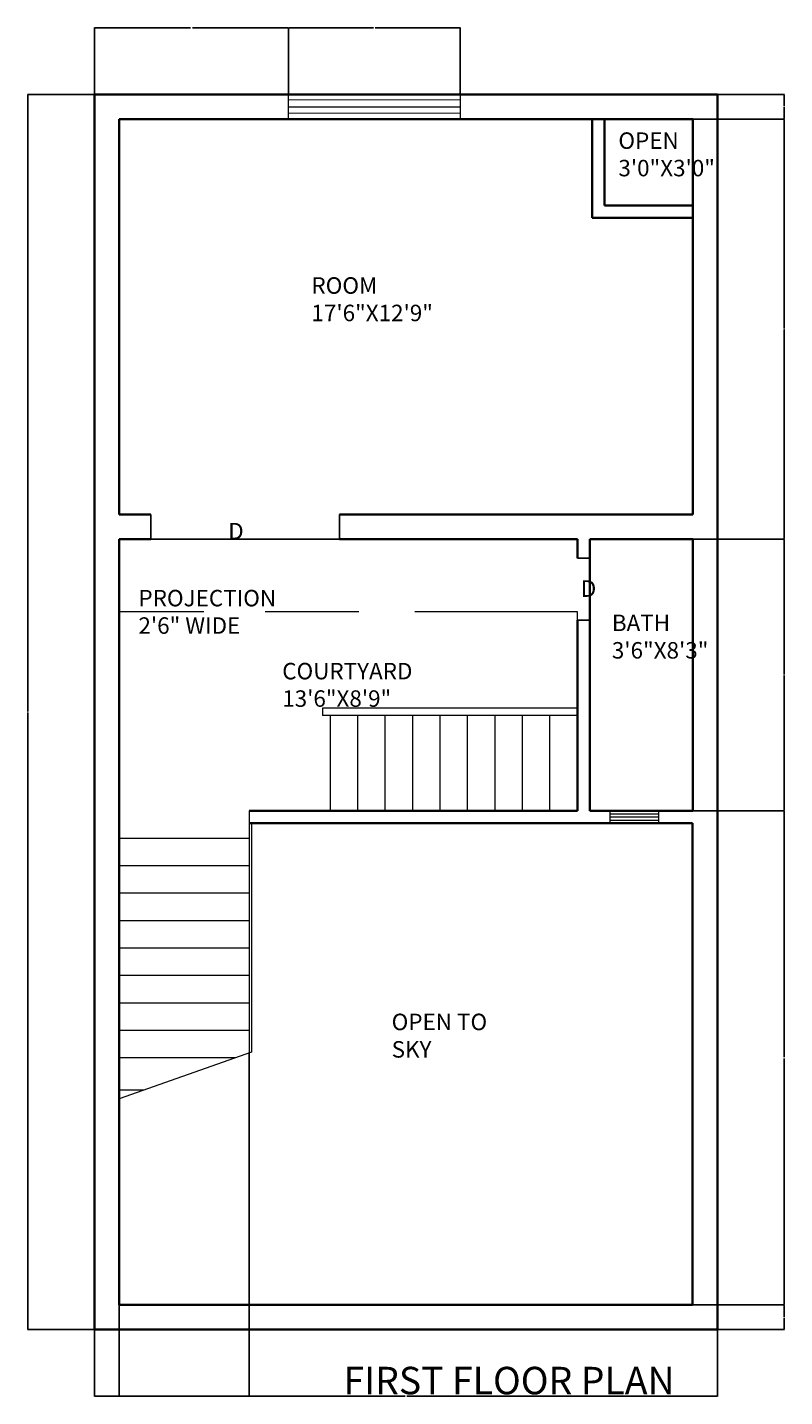
# Model space of a CAD drawing. Units: inches. Extents: x 2673 to 3344, y 1818 to 2362.
# Tile 2 of 2: x 3068 to 3344, y 1819 to 2318. Entities that reach past the tile are written whole.
import ezdxf

# ---------------------------------------------------------------- set-up
doc = ezdxf.new("R2010")
doc.units = ezdxf.units.IN
for name, color, linetype, lineweight in [('A-ANNO-DIMS', 2, 'Continuous', 18), ('A-ANNO-TEXT', 7, 'Continuous', 18), ('A-ANNO-TITL', 7, 'Continuous', 35), ('A-AREA-IDEN', 7, 'Continuous', 18), ('A-DOOR', 3, 'Continuous', 25), ('A-FLOR-PROJ', 8, 'Continuous', 13), ('A-FLOR-STRS', 8, 'Continuous', 18), ('A-GLAZ', 4, 'Continuous', 18), ('A-WALL', 7, 'Continuous', 35)]:
    doc.layers.add(name, color=color, linetype=linetype, lineweight=lineweight)
doc.styles.get("Standard").update_dxf_attribs({"font": 'arial.ttf'})
doc.dimstyles.get("Standard").update_dxf_attribs({"dimtxt": 0.18, "dimasz": 0.18, "dimexe": 0.18, "dimexo": 0.0625, "dimgap": 0.09, "dimtad": 0, "dimtih": 1, "dimtoh": 1, "dimdec": 4, "dimzin": 0, "dimdsep": 46, "dimtxsty": 'Standard', "dimcen": 0.09, "dimadec": 0, "dimazin": 0, "dimtfac": 1, "dimtdec": 4, "dimtofl": 0, "dimtmove": 0, "dimatfit": 3, "dimfxl": 1, "dimtolj": 1, "dimtzin": 0, "dimarcsym": 0})

# ---------------------------------------------------------------- blocks, each defined once
blk = doc.blocks.new('FLOOR-PERIMETER-227X450')
for p, q in [((0, 450), (227, 450)), ((0, 0), (0, 450)), ((227, 450), (227, 0)), ((227, 0), (0, 0))]:
    blk.add_line(p, q)
blk = doc.blocks.new('*D4')
at = {"layer": 'A-ANNO-DIMS', "color": 0, "lineweight": -2, "transparency": 16777216}
for p, q in [((3092.08, 1843.73), (3092.08, 1819.36)), ((3319.08, 1843.73), (3319.08, 1819.36)), ((3092.26, 1819.54), (3205.29, 1819.54)), ((3318.9, 1819.54), (3205.87, 1819.54))]:
    blk.add_line(p, q, dxfattribs=at)
at = {"layer": 'A-ANNO-DIMS', "color": 0, "transparency": 16777216}
for points in [[(3092.26, 1819.57), (3092.26, 1819.51), (3092.08, 1819.54)], [(3318.9, 1819.57), (3318.9, 1819.51), (3319.08, 1819.54)]]:
    blk.add_solid(points, dxfattribs=at)
at = {"layer": 'Defpoints', "color": 0, "transparency": 16777216}
for p in [(3092.08, 1843.79), (3319.08, 1843.79), (3319.08, 1819.54)]:
    blk.add_point(p, dxfattribs=at)
at = {"layer": 'A-ANNO-DIMS', "color": 0, "transparency": 16777216, "insert": (3205.58, 1819.54), "char_height": 0.18, "attachment_point": 5}
blk.add_mtext('\\A1;227', dxfattribs=at)
blk = doc.blocks.new('*D5')
at = {"layer": 'A-ANNO-DIMS', "color": 0, "lineweight": -2, "transparency": 16777216}
for p, q in [((3092.02, 2293.79), (3067.65, 2293.79)), ((3067.83, 2293.61), (3067.83, 2068.98)), ((3067.83, 1843.97), (3067.83, 2068.61)), ((3092.02, 1843.79), (3067.65, 1843.79))]:
    blk.add_line(p, q, dxfattribs=at)
at = {"layer": 'A-ANNO-DIMS', "color": 0, "transparency": 16777216}
for points in [[(3067.8, 2293.61), (3067.86, 2293.61), (3067.83, 2293.79)], [(3067.8, 1843.97), (3067.86, 1843.97), (3067.83, 1843.79)]]:
    blk.add_solid(points, dxfattribs=at)
at = {"layer": 'Defpoints', "color": 0, "transparency": 16777216}
for p in [(3067.83, 2293.79), (3092.08, 2293.79), (3092.08, 1843.79)]:
    blk.add_point(p, dxfattribs=at)
at = {"layer": 'A-ANNO-DIMS', "color": 0, "transparency": 16777216, "insert": (3067.83, 2068.79), "char_height": 0.18, "attachment_point": 5}
blk.add_mtext('\\A1;450', dxfattribs=at)
blk = doc.blocks.new('*D22')
at = {"layer": 'A-ANNO-DIMS', "color": 0, "lineweight": -2, "transparency": 16777216}
for p, q in [((3148.4, 1944.47), (3148.4, 1819.36)), ((3101.08, 1927.78), (3101.08, 1819.36)), ((3101.26, 1819.54), (3124.35, 1819.54)), ((3148.22, 1819.54), (3125.14, 1819.54))]:
    blk.add_line(p, q, dxfattribs=at)
at = {"layer": 'A-ANNO-DIMS', "color": 0, "transparency": 16777216}
for points in [[(3101.26, 1819.57), (3101.26, 1819.51), (3101.08, 1819.54)], [(3148.22, 1819.57), (3148.22, 1819.51), (3148.4, 1819.54)]]:
    blk.add_solid(points, dxfattribs=at)
at = {"layer": 'Defpoints', "color": 0, "transparency": 16777216}
for p in [(3148.4, 1944.54), (3101.08, 1927.84), (3148.4, 1819.54)]:
    blk.add_point(p, dxfattribs=at)
at = {"layer": 'A-ANNO-DIMS', "color": 0, "transparency": 16777216, "insert": (3124.74, 1819.54), "char_height": 0.18, "attachment_point": 5}
blk.add_mtext('\\A1;47.32', dxfattribs=at)
blk = doc.blocks.new('*D23')
at = {"layer": 'A-ANNO-DIMS', "color": 0, "lineweight": -2, "transparency": 16777216}
for p, q in [((3310.09, 1852.79), (3343.51, 1852.79)), ((3343.33, 1852.61), (3343.33, 1848.48)), ((3343.33, 1843.97), (3343.33, 1848.11)), ((3319.14, 1843.79), (3343.51, 1843.79))]:
    blk.add_line(p, q, dxfattribs=at)
at = {"layer": 'A-ANNO-DIMS', "color": 0, "transparency": 16777216}
for points in [[(3343.3, 1852.61), (3343.36, 1852.61), (3343.33, 1852.79)], [(3343.3, 1843.97), (3343.36, 1843.97), (3343.33, 1843.79)]]:
    blk.add_solid(points, dxfattribs=at)
at = {"layer": 'Defpoints', "color": 0, "transparency": 16777216}
for p in [(3310.03, 1852.79), (3343.33, 1852.79), (3319.08, 1843.79)]:
    blk.add_point(p, dxfattribs=at)
at = {"layer": 'A-ANNO-DIMS', "color": 0, "transparency": 16777216, "insert": (3343.33, 1848.29), "char_height": 0.18, "attachment_point": 5}
blk.add_mtext('\\A1;9', dxfattribs=at)
blk = doc.blocks.new('*D24')
at = {"layer": 'A-ANNO-DIMS', "color": 0, "lineweight": -2, "transparency": 16777216}
for p, q in [((3310.14, 2032.8), (3343.51, 2032.8)), ((3343.33, 2032.62), (3343.33, 1942.98)), ((3343.33, 1852.97), (3343.33, 1942.61)), ((3310.09, 1852.79), (3343.51, 1852.79))]:
    blk.add_line(p, q, dxfattribs=at)
at = {"layer": 'A-ANNO-DIMS', "color": 0, "transparency": 16777216}
for points in [[(3343.3, 2032.62), (3343.36, 2032.62), (3343.33, 2032.8)], [(3343.3, 1852.97), (3343.36, 1852.97), (3343.33, 1852.79)]]:
    blk.add_solid(points, dxfattribs=at)
at = {"layer": 'Defpoints', "color": 0, "transparency": 16777216}
for p in [(3310.08, 2032.8), (3343.33, 2032.8), (3310.03, 1852.79)]:
    blk.add_point(p, dxfattribs=at)
at = {"layer": 'A-ANNO-DIMS', "color": 0, "transparency": 16777216, "insert": (3343.33, 1942.8), "char_height": 0.18, "attachment_point": 5}
blk.add_mtext('\\A1;180', dxfattribs=at)
blk = doc.blocks.new('*D25')
at = {"layer": 'A-ANNO-DIMS', "color": 0, "lineweight": -2, "transparency": 16777216}
for p, q in [((3310.14, 2131.8), (3343.51, 2131.8)), ((3343.33, 2131.62), (3343.33, 2082.48)), ((3343.33, 2032.98), (3343.33, 2082.12)), ((3310.14, 2032.8), (3343.51, 2032.8))]:
    blk.add_line(p, q, dxfattribs=at)
at = {"layer": 'A-ANNO-DIMS', "color": 0, "transparency": 16777216}
for points in [[(3343.3, 2131.62), (3343.36, 2131.62), (3343.33, 2131.8)], [(3343.3, 2032.98), (3343.36, 2032.98), (3343.33, 2032.8)]]:
    blk.add_solid(points, dxfattribs=at)
at = {"layer": 'Defpoints', "color": 0, "transparency": 16777216}
for p in [(3310.08, 2131.8), (3343.33, 2131.8), (3310.08, 2032.8)]:
    blk.add_point(p, dxfattribs=at)
at = {"layer": 'A-ANNO-DIMS', "color": 0, "transparency": 16777216, "insert": (3343.33, 2082.3), "char_height": 0.18, "attachment_point": 5}
blk.add_mtext('\\A1;99', dxfattribs=at)
blk = doc.blocks.new('*D26')
at = {"layer": 'A-ANNO-DIMS', "color": 0, "lineweight": -2, "transparency": 16777216}
for p, q in [((3310.14, 2284.79), (3343.51, 2284.79)), ((3343.33, 2284.61), (3343.33, 2208.48)), ((3343.33, 2131.98), (3343.33, 2208.11)), ((3310.14, 2131.8), (3343.51, 2131.8))]:
    blk.add_line(p, q, dxfattribs=at)
at = {"layer": 'A-ANNO-DIMS', "color": 0, "transparency": 16777216}
for points in [[(3343.3, 2284.61), (3343.36, 2284.61), (3343.33, 2284.79)], [(3343.3, 2131.98), (3343.36, 2131.98), (3343.33, 2131.8)]]:
    blk.add_solid(points, dxfattribs=at)
at = {"layer": 'Defpoints', "color": 0, "transparency": 16777216}
for p in [(3310.08, 2284.79), (3343.33, 2284.79), (3310.08, 2131.8)]:
    blk.add_point(p, dxfattribs=at)
at = {"layer": 'A-ANNO-DIMS', "color": 0, "transparency": 16777216, "insert": (3343.33, 2208.3), "char_height": 0.18, "attachment_point": 5}
blk.add_mtext('\\A1;153', dxfattribs=at)
blk = doc.blocks.new('*D27')
at = {"layer": 'A-ANNO-DIMS', "color": 0, "lineweight": -2, "transparency": 16777216}
for p, q in [((3319.14, 2293.79), (3343.51, 2293.79)), ((3343.33, 2293.61), (3343.33, 2289.48)), ((3310.14, 2284.79), (3343.51, 2284.79)), ((3343.33, 2284.97), (3343.33, 2289.11))]:
    blk.add_line(p, q, dxfattribs=at)
at = {"layer": 'A-ANNO-DIMS', "color": 0, "transparency": 16777216}
for points in [[(3343.3, 2293.61), (3343.36, 2293.61), (3343.33, 2293.79)], [(3343.3, 2284.97), (3343.36, 2284.97), (3343.33, 2284.79)]]:
    blk.add_solid(points, dxfattribs=at)
at = {"layer": 'Defpoints', "color": 0, "transparency": 16777216}
for p in [(3319.08, 2293.79), (3343.33, 2293.79), (3310.08, 2284.79)]:
    blk.add_point(p, dxfattribs=at)
at = {"layer": 'A-ANNO-DIMS', "color": 0, "transparency": 16777216, "insert": (3343.33, 2289.29), "char_height": 0.18, "attachment_point": 5}
blk.add_mtext('\\A1;9', dxfattribs=at)
blk = doc.blocks.new('*D28')
at = {"layer": 'A-ANNO-DIMS', "color": 0, "lineweight": -2, "transparency": 16777216}
for p, q in [((3092.08, 2293.86), (3092.08, 2318.22)), ((3092.26, 2318.04), (3127.03, 2318.04)), ((3162.58, 2318.04), (3127.82, 2318.04)), ((3162.76, 2293.86), (3162.76, 2318.22))]:
    blk.add_line(p, q, dxfattribs=at)
at = {"layer": 'A-ANNO-DIMS', "color": 0, "transparency": 16777216}
for points in [[(3092.26, 2318.07), (3092.26, 2318.01), (3092.08, 2318.04)], [(3162.58, 2318.07), (3162.58, 2318.01), (3162.76, 2318.04)]]:
    blk.add_solid(points, dxfattribs=at)
at = {"layer": 'Defpoints', "color": 0, "transparency": 16777216}
for p in [(3162.76, 2318.04), (3092.08, 2293.79), (3162.76, 2293.79)]:
    blk.add_point(p, dxfattribs=at)
at = {"layer": 'A-ANNO-DIMS', "color": 0, "transparency": 16777216, "insert": (3127.42, 2318.04), "char_height": 0.18, "attachment_point": 5}
blk.add_mtext('\\A1;70.68', dxfattribs=at)
blk = doc.blocks.new('*D29')
at = {"layer": 'A-ANNO-DIMS', "color": 0, "lineweight": -2, "transparency": 16777216}
for p, q in [((3162.76, 2293.86), (3162.76, 2318.22)), ((3162.94, 2318.04), (3193.74, 2318.04)), ((3225.18, 2318.04), (3194.39, 2318.04)), ((3225.36, 2293.86), (3225.36, 2318.22))]:
    blk.add_line(p, q, dxfattribs=at)
at = {"layer": 'A-ANNO-DIMS', "color": 0, "transparency": 16777216}
for points in [[(3162.94, 2318.07), (3162.94, 2318.01), (3162.76, 2318.04)], [(3225.18, 2318.07), (3225.18, 2318.01), (3225.36, 2318.04)]]:
    blk.add_solid(points, dxfattribs=at)
at = {"layer": 'Defpoints', "color": 0, "transparency": 16777216}
for p in [(3225.36, 2318.04), (3162.76, 2293.79), (3225.36, 2293.79)]:
    blk.add_point(p, dxfattribs=at)
at = {"layer": 'A-ANNO-DIMS', "color": 0, "transparency": 16777216, "insert": (3194.06, 2318.04), "char_height": 0.18, "attachment_point": 5}
blk.add_mtext('\\A1;62.6', dxfattribs=at)

msp = doc.modelspace()

# ---------------------------------------------------------------- linework, layer by layer
at = {"layer": 'A-DOOR'}
for p, q in [((3112.6344, 2131.7995), (3112.6344, 2140.7995)), ((3181.3427, 2131.7995), (3181.3427, 2140.7995)), ((3112.6344, 2131.7995), (3181.3427, 2131.7995)), ((3268.0279, 2124.8843), (3272.5279, 2124.8843)), ((3268.0279, 2102.2017), (3272.5279, 2102.2017))]:
    msp.add_line(p, q, dxfattribs=at)
at = {"layer": 'A-FLOR-PROJ'}
for p, q in [((3131.8694, 2105.3455), (3101.0804, 2105.3455)), ((3188.3899, 2105.3455), (3154.3017, 2105.3455)), ((3237.0736, 2105.3455), (3208.8429, 2105.3455)), ((3268.0279, 2105.3455), (3237.0736, 2105.3455)), ((3268.0279, 2102.2017), (3268.0279, 2105.3455))]:
    msp.add_line(p, q, dxfattribs=at)
at = {"layer": 'A-FLOR-STRS'}
for p, q in [((3268.0279, 2070.1486), (3175.14, 2070.1486)), ((3175.14, 2070.1486), (3175.14, 2067.5006)), ((3268.0279, 2067.5006), (3175.14, 2067.5006)), ((3178.0279, 2032.7995), (3178.0279, 2067.5006)), ((3188.0279, 2032.7995), (3188.0279, 2067.5006)), ((3198.0279, 2032.7995), (3198.0279, 2067.5006)), ((3208.0279, 2032.7995), (3208.0279, 2067.5006)), ((3218.0279, 2032.7995), (3218.0279, 2067.5006)), ((3228.0279, 2032.7995), (3228.0279, 2067.5006)), ((3238.0279, 2032.7995), (3238.0279, 2067.5006)), ((3248.0279, 2032.7995), (3248.0279, 2067.5006)), ((3258.0279, 2032.7995), (3258.0279, 2067.5006)), ((3148.4041, 2032.7995), (3148.4041, 1944.5366)), ((3149.2926, 2028.2995), (3149.2926, 1944.85)), ((3148.4041, 2022.7553), (3101.0804, 2022.7553)), ((3148.4041, 2012.7553), (3101.0804, 2012.7553)), ((3148.4041, 2002.7553), (3101.0804, 2002.7553)), ((3148.4041, 1992.7553), (3101.0804, 1992.7553)), ((3148.4041, 1982.7553), (3101.0804, 1982.7553)), ((3148.4041, 1972.7553), (3101.0804, 1972.7553)), ((3148.4041, 1962.7553), (3101.0804, 1962.7553)), ((3148.4041, 1952.7553), (3101.0804, 1952.7553)), ((3149.2926, 1944.85), (3101.0804, 1927.8425)), ((3143.3545, 1942.7553), (3101.0804, 1942.7553)), ((3110.1895, 1931.0558), (3101.0804, 1931.0558))]:
    msp.add_line(p, q, dxfattribs=at)
at = {"layer": 'A-GLAZ'}
for p, q in [((3162.7644, 2291.8686), (3225.363, 2291.93)), ((3162.7644, 2289.2936), (3225.363, 2289.2936)), ((3162.7644, 2286.9977), (3225.363, 2287.0505)), ((3279.9327, 2031.7014), (3297.5645, 2031.7014)), ((3279.9327, 2030.5495), (3297.5645, 2030.5495)), ((3279.9327, 2029.387), (3297.5645, 2029.387))]:
    msp.add_line(p, q, dxfattribs=at)
for points in [[(3162.7644, 2293.7936), (3225.363, 2293.7936), (3225.363, 2284.7936), (3162.7644, 2284.7936)], [(3279.9327, 2032.7995), (3297.5645, 2032.7995), (3297.5645, 2028.2995), (3279.9327, 2028.2995)]]:
    msp.add_lwpolyline(points, close=True, dxfattribs=at)
at = {"layer": 'A-WALL'}
for p, q in [((3101.0804, 2284.7936), (3310.0804, 2284.7936)), ((3101.0804, 2140.7995), (3101.0804, 2284.7936)), ((3273.4559, 2248.799), (3273.4559, 2284.7936)), ((3277.9559, 2253.299), (3277.9559, 2284.7936)), ((3310.0804, 2284.7936), (3310.0804, 2140.7995)), ((3309.4559, 2253.299), (3277.9559, 2253.299)), ((3309.4559, 2253.299), (3310.0804, 2253.299)), ((3309.4559, 2248.799), (3273.4559, 2248.799)), ((3309.4559, 2248.799), (3310.0804, 2248.799)), ((3101.0804, 2140.7995), (3112.6344, 2140.7995)), ((3181.3427, 2140.7995), (3310.0804, 2140.7995)), ((3101.0804, 1852.7936), (3101.0804, 2131.7995)), ((3101.0804, 2131.7995), (3112.6344, 2131.7995)), ((3181.3427, 2131.7995), (3268.0279, 2131.7995)), ((3268.0279, 2124.8843), (3268.0279, 2131.7995)), ((3272.5279, 2032.7995), (3272.5279, 2131.7995)), ((3272.5279, 2131.7995), (3310.0804, 2131.7995)), ((3310.0804, 2131.7995), (3310.0804, 2032.7995)), ((3268.0279, 2032.7995), (3268.0279, 2102.2017)), ((3268.0279, 2032.7995), (3148.4041, 2032.7995)), ((3310.0279, 2032.7995), (3272.5279, 2032.7995)), ((3310.0279, 2032.7995), (3310.0804, 2032.7995)), ((3268.0279, 2028.2995), (3148.4041, 2028.2995)), ((3310.0279, 2028.2995), (3268.0279, 2028.2995)), ((3310.0279, 2028.2995), (3310.0279, 1852.7936)), ((3310.0279, 1852.7936), (3101.0804, 1852.7936))]:
    msp.add_line(p, q, dxfattribs=at)

# ---------------------------------------------------------------- block references
at = {"layer": 'A-WALL', "rotation": 180}
msp.add_blockref('FLOOR-PERIMETER-227X450', (3319.0804, 2293.7936), dxfattribs=at)

# ---------------------------------------------------------------- texts
at = {"layer": 'A-ANNO-TEXT', "char_height": 6, "attachment_point": 1}
for s, width, insert in [('D', 13.239528, (3140.7999, 2137.6802)), ('D', 13.239528, (3269.2748, 2116.7486)), ('PROJECTION 2\'6" WIDE ', 53.620126, (3108.0945, 2113.2842))]:
    msp.add_mtext_dynamic_manual_height_columns(s, width=width, gutter_width=12.5, heights=[0], dxfattribs=dict(at, insert=insert))
at = {"layer": 'A-ANNO-TITL', "insert": (3182.789, 1830.2152), "char_height": 10, "attachment_point": 1}
msp.add_mtext_dynamic_manual_height_columns('FIRST FLOOR PLAN ', width=145.417872, gutter_width=12.5, heights=[0], dxfattribs=at)
at = {"layer": 'A-AREA-IDEN', "char_height": 6, "attachment_point": 1}
for s, width, insert in [('OPEN \\P3\'0"X3\'0"', 17.661003, (3282.9682, 2279.9644)), ('ROOM\\P17\'6"X12\'9"', 58.000912, (3171.1277, 2227.1773)), ('BATH\\P3\'6"X8\'3"', 20.788132, (3280.5867, 2104.2645)), ('COURTYARD\\P13\'6"X8\'9"', 34.490092, (3160.4749, 2086.6823)), ('OPEN TO SKY ', 43.395642, (3200.3488, 1958.8809))]:
    msp.add_mtext_dynamic_manual_height_columns(s, width=width, gutter_width=12.5, heights=[0], dxfattribs=dict(at, insert=insert))

# ---------------------------------------------------------------- dimensions: what is measured, and where the dimension line sits
at = {"layer": 'A-ANNO-DIMS'}
for base, p1, p2, override, picture, middle in [((3162.7644, 2318.0436), (3092.0804, 2293.7936), (3162.7644, 2293.7936), {"dimdec": 2, "dimlfac": 1, "dimrnd": 0, "dimzin": 0, "dimdsep": 46, "dimlunit": 2}, '*D28', (3127.4224, 2318.0436)), ((3225.363, 2318.0436), (3162.7644, 2293.7936), (3225.363, 2293.7936), {"dimdec": 1, "dimlfac": 1, "dimrnd": 0, "dimzin": 0, "dimdsep": 46, "dimlunit": 2}, '*D29', (3194.0637, 2318.0436)), ((3148.4041, 1819.5436), (3101.0804, 1927.8425), (3148.4041, 1944.5366), {"dimdec": 2, "dimlfac": 1, "dimrnd": 0, "dimzin": 0, "dimdsep": 46, "dimlunit": 2}, '*D22', (3124.7423, 1819.5436)), ((3319.0804, 1819.5436), (3092.0804, 1843.7936), (3319.0804, 1843.7936), {"dimdec": 0, "dimlfac": 1, "dimrnd": 0, "dimzin": 0, "dimdsep": 46, "dimlunit": 2}, '*D4', (3205.5804, 1819.5436))]:
    dim = msp.add_linear_dim(base=base, p1=p1, p2=p2, dimstyle='Standard', override=override, dxfattribs=at)
    dim.commit()
    dim.dimension.update_dxf_attribs({"geometry": picture, "text_midpoint": middle})
for base, p1, p2, picture, middle in [((3067.8304, 2293.7936), (3092.0804, 1843.7936), (3092.0804, 2293.7936), '*D5', (3067.8304, 2068.7936)), ((3343.3304, 2293.7936), (3310.0804, 2284.7936), (3319.0804, 2293.7936), '*D27', (3343.3304, 2289.2936)), ((3343.3304, 2284.7936), (3310.0804, 2131.7995), (3310.0804, 2284.7936), '*D26', (3343.3304, 2208.2965)), ((3343.3304, 2131.7995), (3310.0804, 2032.7995), (3310.0804, 2131.7995), '*D25', (3343.3304, 2082.2995)), ((3343.3304, 2032.7995), (3310.0279, 1852.7936), (3310.0804, 2032.7995), '*D24', (3343.3304, 1942.7965)), ((3343.3304, 1852.7936), (3319.0804, 1843.7936), (3310.0279, 1852.7936), '*D23', (3343.3304, 1848.2936))]:
    dim = msp.add_linear_dim(base=base, p1=p1, p2=p2, angle=90, dimstyle='Standard', override={"dimdec": 0, "dimlfac": 1, "dimrnd": 0, "dimzin": 0, "dimdsep": 46, "dimlunit": 2}, dxfattribs=at)
    dim.commit()
    dim.dimension.update_dxf_attribs({"geometry": picture, "text_midpoint": middle})

doc.saveas('drawing.dxf')
